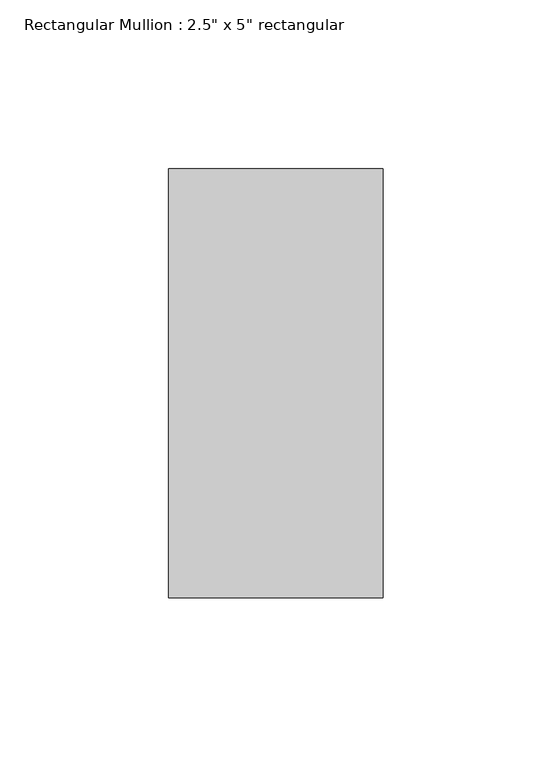
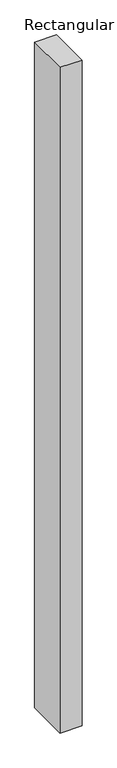
"""IFC4 building model written with IfcOpenShell, lengths in millimetres: member geometry."""

from ifc_helpers import new_model, si_unit, frame, origin, place, context, project, spatial, polyline, outline, extrude, source, transform, mapped, element, save


def member_f95d5bf5(model_context):
    return source(origin(), model_context, "Body", "SweptSolid", [
        extrude(outline(polyline([(31.75, 63.5), (31.75, -63.5), (-31.75, -63.5), (-31.75, 63.5), (31.75, 63.5)])), frame((0.0, 0.0, -2032.0), z_axis=(0.0, 0.0, 1.0), x_axis=(1.0, 0.0, 0.0)), (0.0, 0.0, 1.0), 2032.0),
    ])


if __name__ == "__main__":
    model = new_model("IFC4")
    model_context = context("Model", 3, world=origin())
    ifc_project = project(units=[si_unit("LENGTHUNIT", "METRE", prefix="MILLI")], contexts=[model_context])
    site = spatial("IfcSite", under=ifc_project)
    building = spatial("IfcBuilding", under=site)
    placement = place(None, origin())
    member_shape = member_f95d5bf5(model_context)
    element("IfcMember", 1, ObjectType="Rectangular Mullion : 2.5\" x 5\" rectangular", at=placement, inside=building, context=model_context, shape_type="MappedRepresentation", body=[
        mapped(member_shape, transform((0.0, 0.0, 0.0), x_axis=(1.0, 0.0, 0.0), y_axis=(0.0, 1.0, 0.0), z_axis=(0.0, 0.0, 1.0))),
    ])
    save(model, "model.ifc")

# Revit data of these elements
# Type "Rectangular Mullion : 2.5\" x 5\" rectangular"
#   built-in parameter 1007304 = 0.416667 (stored number, unit not read)
#   built-in parameter 1007301 = 0.104167 (stored number, unit not read)
#   built-in parameter 1007300 = 0.104167 (stored number, unit not read)
